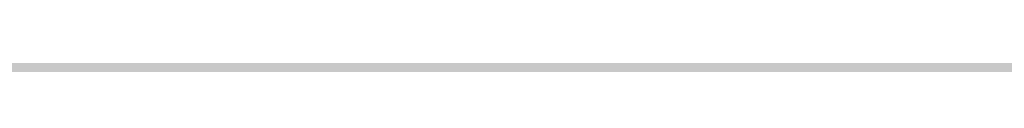
# Model space of a CAD drawing. Units: feet. Extents: x 3168 to 4724, y 827 to 1477.
# Tile 31 of 256: x 3261.901 to 3270.273, y 1099.001 to 1099.015. Entities that reach past the tile are written whole.
import ezdxf

# ---------------------------------------------------------------- set-up
doc = ezdxf.new("R2010")
doc.units = ezdxf.units.FT
doc.layers.add('A-ELEV', color=7, linetype='Continuous', lineweight=35)
doc.layers.add('A-ELEV-PATT', color=8, linetype='Continuous', lineweight=13)

msp = doc.modelspace()

# ---------------------------------------------------------------- hatches: boundary and pattern name
at = {"layer": 'A-ELEV-PATT'}
h = msp.add_hatch(color=256, dxfattribs=at)
h.dxf.hatch_style = 1
edge = h.paths.add_edge_path()
edge.add_ellipse((3552.9058, 979.2201), major_axis=(36.7449, 0), ratio=0.4848485, start_angle=0, end_angle=360)
edge = h.paths.add_edge_path()
edge.add_ellipse((3559.8916, 929.2523), major_axis=(36.7449, 0), ratio=0.4848485, start_angle=0, end_angle=360)
edge = h.paths.add_edge_path()
edge.add_line((3299.3168, 1198.6061), (3479.9167, 1198.6061))
edge.add_line((3479.9167, 1198.6061), (3479.9167, 1209.8686))
edge.add_spline(control_points=[(3479.9167, 1209.8686), (3464.3012, 1209.8686), (3448.6856, 1209.8686), (3410.9491, 1209.8686), (3388.8282, 1209.8686), (3355.6469, 1209.8686), (3344.5864, 1209.8686), (3327.9957, 1209.8686), (3322.4655, 1209.8686), (3314.1702, 1209.8686), (3311.4051, 1209.8686), (3307.2574, 1209.8686), (3305.8748, 1209.8686), (3303.801, 1209.8686), (3303.1097, 1209.8686), (3302.0728, 1209.8686), (3301.7272, 1209.8686), (3301.2087, 1209.8686), (3301.0359, 1209.8686), (3300.7767, 1209.8686), (3300.6903, 1209.8686), (3300.5606, 1209.8686), (3300.5174, 1209.8686), (3300.4526, 1209.8686), (3300.431, 1209.8686), (3300.3986, 1209.8686), (3300.3878, 1209.8686), (3300.3662, 1209.8686), (3300.3457, 1209.8686), (3300.3455, 1209.8686), (3300.3455, 1209.8686), (3300.3433, 1209.8686), (3300.3411, 1209.8686), (3300.3379, 1209.8686), (3300.3368, 1209.8686), (3300.3339, 1209.8686), (3300.3321, 1209.8686), (3300.3255, 1209.8686), (3300.3207, 1209.8686), (3300.3109, 1209.8686), (3300.306, 1209.8686), (3300.2905, 1209.8686), (3300.28, 1209.8686), (3300.2324, 1209.8688), (3300.1953, 1209.869), (3299.9511, 1209.8706), (3299.7448, 1209.8743), (3299.4368, 1209.8833), (3299.3344, 1209.8868), (3299.1811, 1209.8929), (3299.13, 1209.8951), (3298.6522, 1209.9168), (3298.2295, 1209.9457), (3297.6016, 1210.0024), (3297.3934, 1210.0235), (3297.0827, 1210.0583), (3296.9793, 1210.0705), (3296.293, 1210.1549), (3295.7181, 1210.2434), (3294.8687, 1210.3989), (3294.5877, 1210.4545), (3294.1693, 1210.5433), (3294.0304, 1210.5739), (3291.7071, 1211.1012), (3289.6536, 1211.8134), (3285.7763, 1213.564), (3283.9514, 1214.6035), (3280.5122, 1216.9801), (3278.8972, 1218.3176), (3276.3799, 1220.8295), (3275.416, 1221.9177), (3274.0393, 1223.7077), (3273.581, 1224.3495), (3273.1432, 1225.0163)], knot_values=[39.119033, 39.119033, 39.119033, 39.119033, 39.286353, 39.286353, 39.523379, 39.523379, 39.641892, 39.641892, 39.701148, 39.701148, 39.730777, 39.730777, 39.745591, 39.745591, 39.752998, 39.752998, 39.756701, 39.756701, 39.758553, 39.758553, 39.759479, 39.759479, 39.759942, 39.759942, 39.760173, 39.760173, 39.760289, 39.760289, 39.760405, 39.760405, 39.760463, 39.760463, 39.763389, 39.763389, 39.764851, 39.764851, 39.767304, 39.767304, 39.773825, 39.773825, 39.78057, 39.78057, 39.79477, 39.79477, 39.845194, 39.845194, 40.126715, 40.126715, 40.267476, 40.267476, 40.337856, 40.337856, 40.927023, 40.927023, 41.221606, 41.221606, 41.368898, 41.368898, 42.202622, 42.202622, 42.619485, 42.619485, 42.827916, 42.827916, 46.118323, 46.118323, 49.408731, 49.408731, 52.699139, 52.699139, 54.927489, 54.927489, 56.104228, 56.104228, 56.104228, 56.104228], weights=[1, 1, 1, 1, 1, 1, 1, 1, 1, 1, 1, 1, 1, 1, 1, 1, 1, 1, 1, 1, 1, 1, 1, 1, 1, 1, 1, 1, 1, 1, 1, 1, 1, 1, 1, 1, 1, 1, 1, 1, 1, 1, 1, 1, 1, 1, 1, 1, 1, 1, 1, 1, 1, 1, 1, 1, 1, 1, 1, 1, 1, 1, 1, 1, 1, 1, 1, 1, 1, 1, 1, 1, 1, 1], degree=3, periodic=0)
edge.add_line((3273.1432, 1225.0163), (3273.1432, 1099.0163))
edge.add_line((3273.1432, 1099.0163), (3299.3168, 1099.0163))
edge.add_line((3299.3168, 1099.0163), (3299.3168, 1198.6061))
edge = h.paths.add_edge_path()
edge.add_line((3304.7584, 1324.1581), (3479.9167, 1324.1581))
edge.add_line((3479.9167, 1324.1581), (3479.9167, 1335.7146))
edge.add_line((3479.9167, 1335.7146), (3269.1616, 1335.7146))
edge.add_spline(control_points=[(3269.1616, 1335.7146), (3264.0242, 1335.7146), (3258.3641, 1328.9582), (3259.2643, 1323.9003)], knot_values=[0, 0, 0, 0, 15.412191, 15.412191, 15.412191, 15.412191], degree=3, periodic=0)
edge.add_line((3259.2643, 1323.9003), (3265.5168, 1288.7691))
edge.add_line((3265.5168, 1288.7691), (3275.2651, 1261.5456))
edge.add_line((3275.2651, 1261.5456), (3304.7584, 1261.5456))
edge.add_line((3304.7584, 1261.5456), (3304.7584, 1324.1581))
h = msp.add_hatch(color=256, dxfattribs=at)
h.dxf.hatch_style = 1
h.paths.add_polyline_path([(3384.5252, 1099.0163), (3335.0292, 1099.0163), (3299.3168, 1099.0163), (3273.1432, 1099.0163), (3217.5654, 1099.0163), (3168.0693, 827.1163), (3335.0292, 827.1163)])

# ---------------------------------------------------------------- linework, layer by layer
at = {"layer": 'A-ELEV'}
msp.add_open_spline([(3808.5202, 1099.0163), (3808.5202, 1141.4132), (3808.5202, 1183.8102), (3808.5202, 1226.6353), (3808.5202, 1227.0636), (3808.5202, 1227.4918), (3811.4919, 1248.9947), (3814.4635, 1270.4975), (3817.4652, 1292.2176), (3817.4952, 1292.4348), (3817.5253, 1292.652), (3817.5728, 1310.1067), (3817.6203, 1327.5615), (3817.6679, 1345.0163), (3817.6679, 1345.458), (3817.6679, 1345.8996), (3817.6679, 1346.456), (3817.6679, 1346.5708), (3817.6679, 1346.7529), (3817.6679, 1346.8201), (3817.6679, 1346.9349), (3817.6679, 1346.9823), (3817.6679, 1347.0386), (3817.6679, 1347.0474), (3817.6679, 1347.0737), (3817.6679, 1347.0593), (3817.6679, 1347.0615), (3817.6679, 1347.0627), (3817.6679, 1347.066), (3817.6679, 1347.0683), (3817.6679, 1347.075), (3817.6679, 1347.0795), (3817.6678, 1347.0929), (3817.6678, 1347.1019), (3817.6678, 1347.1288), (3817.6677, 1347.1467), (3817.6674, 1347.2004), (3817.6672, 1347.2362), (3817.6661, 1347.3434), (3817.665, 1347.4147), (3817.6608, 1347.6281), (3817.6566, 1347.7697), (3817.64, 1348.1925), (3817.6235, 1348.4716), (3817.5591, 1349.3001), (3817.4961, 1349.8406), (3817.2554, 1351.4242), (3817.0263, 1352.4288), (3816.3069, 1354.8889), (3815.7437, 1356.2687), (3814.464, 1358.8192), (3813.7464, 1359.991), (3812.1958, 1362.1723), (3811.3622, 1363.1821), (3809.5888, 1365.069), (3808.6488, 1365.9461), (3806.6543, 1367.5796), (3805.5997, 1368.3362), (3803.3529, 1369.7223), (3802.1605, 1370.3524), (3799.6008, 1371.4536), (3798.2327, 1371.9255), (3795.2801, 1372.6346), (3793.6931, 1372.8721), (3791.8694, 1372.9265), (3791.7409, 1372.9292), (3791.3534, 1372.9341), (3791.0927, 1372.9329), (3790.3041, 1372.9151), (3789.7695, 1372.8842), (3789.2092, 1372.8302), (3789.1906, 1372.8284), (3789.1349, 1372.8229), (3789.0977, 1372.8191), (3789.0484, 1372.814), (3789.0364, 1372.8127), (3789.0003, 1372.8089), (3788.9761, 1372.8063), (3788.9494, 1372.8034), (3788.9468, 1372.8031), (3788.9426, 1372.8027), (3788.941, 1372.8025), (3788.9386, 1372.8022), (3788.9378, 1372.8021), (3788.9354, 1372.8019), (3788.8675, 1372.7944), (3788.7569, 1372.7822), (3788.7015, 1372.7761), (3788.5355, 1372.7579), (3788.4249, 1372.7457), (3788.0929, 1372.7092), (3787.8715, 1372.6848), (3787.2075, 1372.6118), (3786.7648, 1372.5631), (3785.4368, 1372.417), (3784.5515, 1372.3196), (3781.8954, 1372.0274), (3780.1247, 1371.8327), (3774.8126, 1371.2483), (3771.2713, 1370.8587), (3760.6471, 1369.69), (3753.5643, 1368.9109), (3732.316, 1366.5735), (3718.1504, 1365.0152), (3694.0068, 1362.3593), (3684.0287, 1361.2617), (3674.0506, 1360.1641), (3664.6007, 1360.1641), (3655.1508, 1360.1641), (3626.8011, 1360.1641), (3607.9013, 1360.1641), (3551.2019, 1360.1641), (3513.4023, 1360.1641), (3467.7252, 1360.1641), (3459.8476, 1360.1641), (3436.2149, 1360.1641), (3420.4597, 1360.1641), (3373.1943, 1360.1641), (3341.6839, 1360.1641), (3302.8482, 1360.1641), (3295.5227, 1360.1641), (3286.0383, 1360.1641), (3283.8794, 1360.1641), (3277.4026, 1360.1641), (3273.0848, 1360.1641), (3267.7329, 1360.1641), (3266.6988, 1360.1641), (3263.5965, 1360.1641), (3261.5284, 1360.1641), (3259.2369, 1360.1641), (3259.0137, 1360.1641), (3258.344, 1360.1641), (3257.8975, 1360.1641), (3257.431, 1360.1641), (3257.411, 1360.1641), (3257.3706, 1360.1641), (3257.3755, 1360.1641), (3257.3746, 1360.1641), (3257.3739, 1360.1641), (3257.372, 1360.1641), (3257.3706, 1360.1641), (3257.3667, 1360.1641), (3257.364, 1360.1641), (3257.3561, 1360.1641), (3257.3508, 1360.164), (3257.335, 1360.164), (3257.3244, 1360.164), (3257.2928, 1360.1639), (3257.2717, 1360.1638), (3257.2084, 1360.1634), (3257.1663, 1360.163), (3257.0402, 1360.1614), (3256.9563, 1360.1598), (3256.7055, 1360.1534), (3256.5392, 1360.147), (3256.0436, 1360.1219), (3255.7173, 1360.0971), (3254.7524, 1360.0005), (3254.128, 1359.9065), (3252.1801, 1359.5253), (3250.9416, 1359.144), (3248.6702, 1358.2433), (3247.6357, 1357.7238), (3245.7326, 1356.6035), (3244.8634, 1356.0021), (3243.2531, 1354.7429), (3242.512, 1354.0847), (3240.7511, 1352.3448), (3239.801, 1351.2296), (3238.0878, 1348.8724), (3237.3247, 1347.6304), (3235.9825, 1344.9716), (3235.4022, 1343.5549), (3234.5911, 1340.8155), (3234.3109, 1339.5435), (3233.9765, 1336.8026), (3233.9221, 1335.3309), (3234.1489, 1332.5913), (3234.3495, 1331.3672), (3234.7199, 1329.9994), (3234.7524, 1329.8834), (3234.8536, 1329.5348), (3234.9259, 1329.3017), (3235.0248, 1329.0026), (3235.0469, 1328.9369), (3235.0776, 1328.8472), (3235.0859, 1328.8232), (3235.1109, 1328.7511), (3235.1278, 1328.703), (3235.148, 1328.6462), (3235.1511, 1328.6376), (3235.1561, 1328.6235), (3235.1581, 1328.618), (3235.1602, 1328.612), (3235.1656, 1328.5969), (3235.1801, 1328.5565), (3235.1903, 1328.5281), (3235.2208, 1328.4429), (3235.2411, 1328.3862), (3235.3021, 1328.2159), (3235.3427, 1328.1023), (3235.4647, 1327.7617), (3235.546, 1327.5346), (3235.79, 1326.8534), (3235.9526, 1326.3992), (3236.4405, 1325.0367), (3236.7657, 1324.1284), (3237.7415, 1321.4034), (3238.392, 1319.5868), (3240.3435, 1314.1369), (3241.6445, 1310.5036), (3245.5476, 1299.6037), (3248.1496, 1292.3371), (3255.9557, 1270.5374), (3261.1598, 1256.0042), (3267.3876, 1238.612), (3268.4114, 1235.7529), (3269.5104, 1232.6839), (3269.5856, 1232.4739), (3269.7066, 1232.1359), (3269.7524, 1232.0079), (3269.8273, 1231.7987), (3269.8564, 1231.7176), (3269.9063, 1231.5781), (3269.9272, 1231.5198), (3269.9725, 1231.3934), (3269.9968, 1231.3254), (3270.0265, 1231.2425), (3270.0318, 1231.2277), (3270.0403, 1231.204), (3270.0392, 1231.207), (3270.0394, 1231.2066), (3270.0394, 1231.2064), (3270.0396, 1231.2058), (3270.0398, 1231.2055), (3270.0402, 1231.2043), (3270.0404, 1231.2036), (3270.0413, 1231.2013), (3270.0418, 1231.1998), (3270.0434, 1231.1953), (3270.0445, 1231.1922), (3270.0478, 1231.1832), (3270.0499, 1231.1771), (3270.0564, 1231.159), (3270.0608, 1231.147), (3270.0739, 1231.1108), (3270.0826, 1231.0867), (3270.1089, 1231.0144), (3270.1266, 1230.9663), (3270.1799, 1230.8225), (3270.2159, 1230.7269), (3270.3253, 1230.4415), (3270.4, 1230.2528), (3270.6292, 1229.6914), (3270.7889, 1229.3235), (3271.2865, 1228.2383), (3271.6431, 1227.5398), (3272.7759, 1225.5153), (3273.6142, 1224.2605), (3275.416, 1221.9177), (3276.3799, 1220.8295), (3278.8972, 1218.3176), (3280.5122, 1216.9801), (3283.9514, 1214.6035), (3285.7763, 1213.564), (3289.6536, 1211.8134), (3291.7071, 1211.1012), (3294.0304, 1210.5739), (3294.1693, 1210.5433), (3294.5877, 1210.4545), (3294.8687, 1210.3989), (3295.7181, 1210.2434), (3296.293, 1210.1549), (3296.9793, 1210.0705), (3297.0827, 1210.0583), (3297.3934, 1210.0235), (3297.6016, 1210.0024), (3298.2295, 1209.9457), (3298.6522, 1209.9168), (3299.13, 1209.8951), (3299.1811, 1209.8929), (3299.3344, 1209.8868), (3299.4368, 1209.8833), (3299.7448, 1209.8743), (3299.9511, 1209.8706), (3300.1953, 1209.869), (3300.2324, 1209.8688), (3300.28, 1209.8686), (3300.2905, 1209.8686), (3300.306, 1209.8686), (3300.3109, 1209.8686), (3300.3207, 1209.8686), (3300.3255, 1209.8686), (3300.3321, 1209.8686), (3300.3339, 1209.8686), (3300.3368, 1209.8686), (3300.3379, 1209.8686), (3300.3411, 1209.8686), (3300.3433, 1209.8686), (3300.3455, 1209.8686), (3300.3455, 1209.8686), (3300.3457, 1209.8686), (3300.3662, 1209.8686), (3300.3878, 1209.8686), (3300.3986, 1209.8686), (3300.431, 1209.8686), (3300.4526, 1209.8686), (3300.5174, 1209.8686), (3300.5606, 1209.8686), (3300.6903, 1209.8686), (3300.7767, 1209.8686), (3301.0359, 1209.8686), (3301.2087, 1209.8686), (3301.7272, 1209.8686), (3302.0728, 1209.8686), (3303.1097, 1209.8686), (3303.801, 1209.8686), (3305.8748, 1209.8686), (3307.2574, 1209.8686), (3311.4051, 1209.8686), (3314.1702, 1209.8686), (3322.4655, 1209.8686), (3327.9957, 1209.8686), (3344.5864, 1209.8686), (3355.6469, 1209.8686), (3388.8282, 1209.8686), (3410.9491, 1209.8686), (3477.3119, 1209.8686), (3521.5537, 1209.8686), (3566.8362, 1209.8686), (3567.8769, 1209.8686), (3570.999, 1209.8686), (3573.0804, 1209.8686), (3575.7814, 1209.8686), (3576.4009, 1209.8686), (3577.2958, 1209.8686), (3577.5712, 1209.8686), (3578.3971, 1209.8686), (3578.9478, 1209.8686), (3579.7565, 1209.8686), (3580.0145, 1209.8686), (3580.3427, 1209.8686), (3580.3269, 1209.8686), (3580.3272, 1209.8686), (3580.3273, 1209.8686), (3580.3278, 1209.8686), (3580.3281, 1209.8686), (3580.329, 1209.8686), (3580.3296, 1209.8686), (3580.3314, 1209.8686), (3580.3327, 1209.8686), (3580.3363, 1209.8686), (3580.3388, 1209.8686), (3580.3461, 1209.8686), (3580.351, 1209.8686), (3580.3657, 1209.8685), (3580.3754, 1209.8685), (3580.4048, 1209.8684), (3580.4244, 1209.8684), (3580.4832, 1209.8681), (3580.5224, 1209.8678), (3580.6404, 1209.8666), (3580.7192, 1209.8655), (3580.9563, 1209.8608), (3581.1152, 1209.8561), (3581.5942, 1209.8372), (3581.9164, 1209.8183), (3582.8899, 1209.7424), (3583.548, 1209.6662), (3585.5318, 1209.3606), (3586.8672, 1209.0539), (3589.4715, 1208.2525), (3590.7402, 1207.7579), (3591.9955, 1207.1588), (3592.0578, 1207.1287), (3592.2442, 1207.038), (3592.3677, 1206.9766), (3592.7353, 1206.7904), (3592.9768, 1206.6631), (3593.2445, 1206.5164), (3593.2747, 1206.4998), (3593.3651, 1206.4498), (3593.4251, 1206.4163), (3593.6043, 1206.3153), (3593.7227, 1206.2472), (3593.8572, 1206.1684), (3593.8744, 1206.1583), (3593.9257, 1206.128), (3593.9599, 1206.1078), (3594.0621, 1206.0469), (3594.1298, 1206.0061), (3594.2084, 1205.9582), (3594.2197, 1205.9513), (3594.2534, 1205.9307), (3594.2758, 1205.9169), (3594.343, 1205.8755), (3594.3876, 1205.8479), (3594.4336, 1205.819), (3594.4353, 1205.818), (3594.4402, 1205.8149), (3594.4435, 1205.8129), (3594.4471, 1205.8106), (3594.4475, 1205.8103), (3594.4487, 1205.8096), (3594.4495, 1205.8091), (3594.4504, 1205.8086), (3594.4505, 1205.8085), (3594.4506, 1205.8084), (3594.4674, 1205.7979), (3594.4933, 1205.7817), (3594.5062, 1205.7736), (3594.545, 1205.7492), (3594.5709, 1205.733), (3594.6485, 1205.6844), (3594.7002, 1205.652), (3594.8554, 1205.5547), (3594.9589, 1205.4898), (3595.2694, 1205.2953), (3595.4763, 1205.1656), (3596.0972, 1204.7765), (3596.5111, 1204.5171), (3597.7528, 1203.7388), (3598.5807, 1203.22), (3601.0642, 1201.6636), (3602.7198, 1200.6259), (3607.6868, 1197.513), (3610.9981, 1195.4377), (3620.932, 1189.2119), (3627.5546, 1185.0614), (3647.4225, 1172.6097), (3660.6678, 1164.3086), (3700.4035, 1139.4053), (3726.894, 1122.8031), (3757.2057, 1103.8061), (3761.027, 1101.4112), (3764.8482, 1099.0163), (3745.3283, 1099.0163), (3725.8083, 1099.0163), (3706.2884, 1099.0163), (3706.2884, 1108.4532), (3706.2884, 1117.8902), (3706.2884, 1127.3271), (3710.7508, 1127.3271), (3715.2131, 1127.3271), (3719.6755, 1127.3271)], degree=3, knots=[0, 0, 0, 0, 0.982037, 0.982037, 0.991957, 0.991957, 0.991957, 1.966522, 1.966522, 1.976367, 1.976367, 1.976367, 2.976367, 2.976367, 2.976367, 3.00169, 3.00169, 3.008272, 3.008272, 3.012129, 3.012129, 3.014851, 3.014851, 3.015353, 3.015353, 3.016359, 3.016359, 3.017365, 3.017365, 3.019376, 3.019376, 3.023398, 3.023398, 3.031442, 3.031442, 3.047531, 3.047531, 3.079708, 3.079708, 3.144063, 3.144063, 3.272772, 3.272772, 3.53019, 3.53019, 4.045026, 4.045026, 5.074698, 5.074698, 6.700878, 6.700878, 8.327058, 8.327058, 9.953238, 9.953238, 11.579418, 11.579418, 13.205598, 13.205598, 14.831778, 14.831778, 16.457958, 16.457958, 18.084138, 18.084138, 18.206872, 18.206872, 18.45234, 18.45234, 18.943275, 18.943275, 18.960093, 18.960093, 18.993729, 18.993729, 19.00461, 19.00461, 19.026374, 19.026374, 19.028737, 19.028737, 19.03018, 19.03018, 19.030897, 19.030897, 19.032332, 19.032332, 19.033766, 19.033766, 19.036636, 19.036636, 19.042374, 19.042374, 19.053851, 19.053851, 19.076805, 19.076805, 19.122714, 19.122714, 19.21453, 19.21453, 19.398163, 19.398163, 19.765429, 19.765429, 20.024128, 20.024128, 20.024128, 20.092031, 20.092031, 20.227836, 20.227836, 20.499446, 20.499446, 20.556051, 20.556051, 20.66926, 20.66926, 20.895678, 20.895678, 20.948316, 20.948316, 20.963829, 20.963829, 20.994855, 20.994855, 21.002285, 21.002285, 21.017146, 21.017146, 21.01875, 21.01875, 21.021959, 21.021959, 21.022102, 21.022102, 21.022249, 21.022249, 21.022708, 21.022708, 21.023627, 21.023627, 21.025464, 21.025464, 21.029138, 21.029138, 21.036486, 21.036486, 21.051183, 21.051183, 21.080575, 21.080575, 21.139361, 21.139361, 21.256932, 21.256932, 21.492073, 21.492073, 21.962356, 21.962356, 23.01002, 23.01002, 24.057684, 24.057684, 25.105348, 25.105348, 26.153011, 26.153011, 27.776787, 27.776787, 29.400562, 29.400562, 31.024337, 31.024337, 32.278801, 32.278801, 33.533265, 33.533265, 34.467568, 34.467568, 34.553971, 34.553971, 34.726776, 34.726776, 34.775309, 34.775309, 34.793079, 34.793079, 34.82862, 34.82862, 34.834979, 34.834979, 34.839039, 34.839039, 34.839411, 34.839411, 34.840285, 34.840285, 34.842034, 34.842034, 34.845531, 34.845531, 34.852525, 34.852525, 34.866512, 34.866512, 34.894488, 34.894488, 34.950439, 34.950439, 35.062342, 35.062342, 35.286147, 35.286147, 35.733758, 35.733758, 35.821815, 35.821815, 35.828283, 35.828283, 35.832225, 35.832225, 35.834724, 35.834724, 35.836521, 35.836521, 35.838617, 35.838617, 35.839073, 35.839073, 35.839345, 35.839345, 35.839617, 35.839617, 35.840161, 35.840161, 35.841249, 35.841249, 35.843425, 35.843425, 35.847778, 35.847778, 35.856482, 35.856482, 35.873891, 35.873891, 35.908709, 35.908709, 35.978345, 35.978345, 36.117617, 36.117617, 36.396161, 36.396161, 36.953248, 36.953248, 38.067423, 38.067423, 40.295772, 40.295772, 42.524122, 42.524122, 45.81453, 45.81453, 49.104937, 49.104937, 52.395345, 52.395345, 52.603776, 52.603776, 53.020639, 53.020639, 53.854363, 53.854363, 54.001655, 54.001655, 54.296238, 54.296238, 54.885405, 54.885405, 54.955785, 54.955785, 55.096546, 55.096546, 55.378067, 55.378067, 55.42849, 55.42849, 55.442691, 55.442691, 55.449436, 55.449436, 55.455957, 55.455957, 55.458409, 55.458409, 55.459872, 55.459872, 55.462798, 55.462798, 55.462856, 55.462856, 55.462972, 55.462972, 55.463088, 55.463088, 55.463319, 55.463319, 55.463782, 55.463782, 55.464708, 55.464708, 55.46656, 55.46656, 55.470263, 55.470263, 55.47767, 55.47767, 55.492484, 55.492484, 55.522112, 55.522112, 55.581369, 55.581369, 55.699882, 55.699882, 55.936907, 55.936907, 56.410959, 56.410959, 56.42211, 56.42211, 56.444413, 56.444413, 56.451051, 56.451051, 56.454001, 56.454001, 56.459901, 56.459901, 56.462666, 56.462666, 56.463418, 56.463418, 56.464171, 56.464171, 56.465675, 56.465675, 56.468684, 56.468684, 56.474702, 56.474702, 56.486738, 56.486738, 56.51081, 56.51081, 56.558955, 56.558955, 56.655243, 56.655243, 56.847821, 56.847821, 57.232975, 57.232975, 58.003284, 58.003284, 59.543901, 59.543901, 62.625137, 62.625137, 68.787607, 68.787607, 74.950078, 74.950078, 75.27336, 75.27336, 75.919923, 75.919923, 77.213051, 77.213051, 77.377769, 77.377769, 77.707206, 77.707206, 78.366079, 78.366079, 78.462532, 78.462532, 78.655436, 78.655436, 79.041245, 79.041245, 79.105735, 79.105735, 79.234714, 79.234714, 79.492672, 79.492672, 79.502197, 79.502197, 79.521249, 79.521249, 79.523534, 79.523534, 79.528103, 79.528103, 79.528682, 79.528682, 79.528885, 79.528885, 79.529089, 79.529089, 79.529495, 79.529495, 79.530308, 79.530308, 79.531935, 79.531935, 79.535187, 79.535187, 79.541693, 79.541693, 79.554704, 79.554704, 79.580725, 79.580725, 79.632769, 79.632769, 79.736856, 79.736856, 79.94503, 79.94503, 80.361377, 80.361377, 80.421435, 80.421435, 80.421435, 81.421435, 81.421435, 81.421435, 82.421435, 82.421435, 82.421435, 83.421435, 83.421435, 83.421435, 83.421435], dxfattribs=at)

doc.saveas('drawing.dxf')
